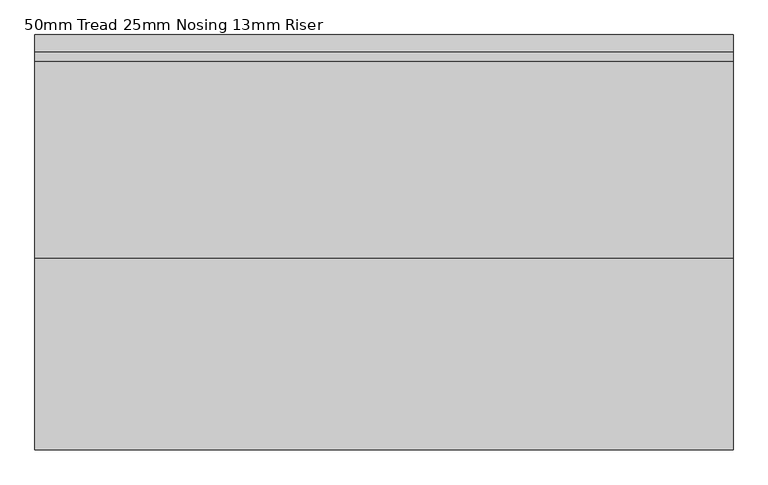
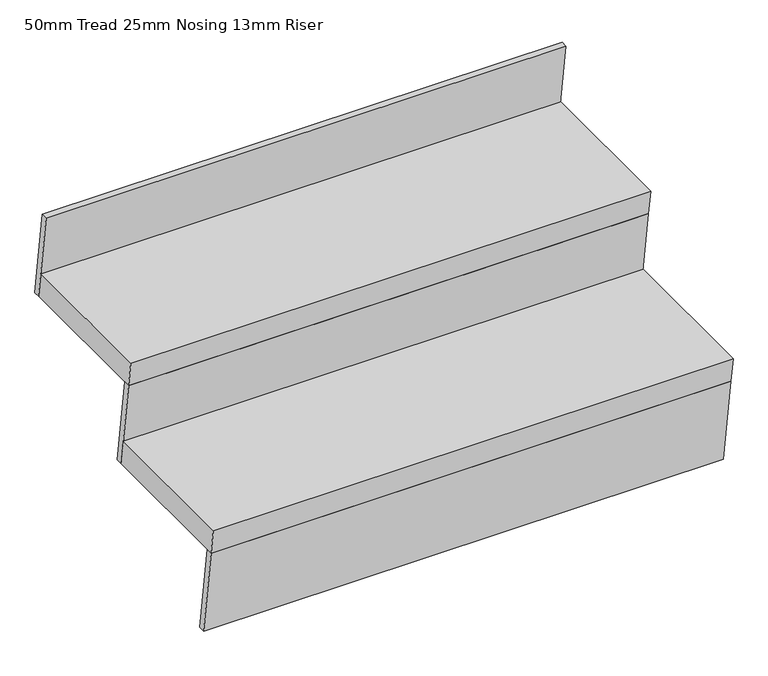
"""IFC4 building model written with IfcOpenShell, lengths in millimetres: stair flight geometry, 50mm Tread 25mm Nosing 13mm Riser."""

from ifc_helpers import new_model, si_unit, frame, origin, place, context, project, spatial, polyline, outline, extrude, source, transform, mapped, element, save


def stair_flight_50mm_tread_25mm_nosing_13mm_riser_775a8025(model_context):
    return source(origin(), model_context, "Body", "SweptSolid", [
        extrude(outline(polyline([(7333.8660835, 1217.3913043), (7633.8660835, 1217.3913043), (7641.0535835, 1167.3913043), (7341.0535835, 1167.3913043), (7333.8660835, 1217.3913043)])), frame((-12602.0787807, 0.0, 0.0), z_axis=(1.0, 0.0, 0.0), x_axis=(0.0, 1.0, 0.0)), (0.0, 0.0, 1.0), 1000.0257812),
        extrude(outline(polyline([(7341.0535835, 1167.3913043), (7353.6820735, 1167.3913043), (7378.6820735, 993.4782609), (7366.0535835, 993.4782609), (7341.0535835, 1167.3913043)])), frame((-12602.0787807, 0.0, 0.0), z_axis=(1.0, 0.0, 0.0), x_axis=(0.0, 1.0, 0.0)), (0.0, 0.0, 1.0), 1000.0257813),
        extrude(outline(polyline([(7616.0535835, 1341.3043478), (7628.6820735, 1341.3043478), (7653.6820735, 1167.3913043), (7641.0535835, 1167.3913043), (7616.0535835, 1341.3043478)])), frame((-12602.0787807, 0.0, 0.0), z_axis=(1.0, 0.0, 0.0), x_axis=(0.0, 1.0, 0.0)), (0.0, 0.0, 1.0), 1000.0257813),
        extrude(outline(polyline([(7891.0535835, 1515.2173913), (7903.6820735, 1515.2173913), (7928.6820735, 1341.3043478), (7916.0535835, 1341.3043478), (7891.0535835, 1515.2173913)])), frame((-12602.0787807, 0.0, 0.0), z_axis=(1.0, 0.0, 0.0), x_axis=(0.0, 1.0, 0.0)), (0.0, 0.0, 1.0), 1000.0257813),
        extrude(outline(polyline([(7608.8660835, 1391.3043478), (7908.8660835, 1391.3043478), (7916.0535835, 1341.3043478), (7616.0535835, 1341.3043478), (7608.8660835, 1391.3043478)])), frame((-12602.0787807, 0.0, 0.0), z_axis=(1.0, 0.0, 0.0), x_axis=(0.0, 1.0, 0.0)), (0.0, 0.0, 1.0), 1000.0257812),
    ])


if __name__ == "__main__":
    model = new_model("IFC4")
    model_context = context("Model", 3, world=origin())
    ifc_project = project(units=[si_unit("LENGTHUNIT", "METRE", prefix="MILLI")], contexts=[model_context])
    site = spatial("IfcSite", under=ifc_project)
    building = spatial("IfcBuilding", under=site)
    placement = place(None, origin())
    stair_flight_50mm_tread_25mm_nosing_13mm_riser_shape = stair_flight_50mm_tread_25mm_nosing_13mm_riser_775a8025(model_context)
    element("IfcStairFlight", 1, ObjectType="50mm Tread 25mm Nosing 13mm Riser", at=placement, inside=building, context=model_context, shape_type="MappedRepresentation", body=[
        mapped(stair_flight_50mm_tread_25mm_nosing_13mm_riser_shape, transform((0.0, 0.0, 0.0), x_axis=(1.0, 0.0, 0.0), y_axis=(0.0, 1.0, 0.0), z_axis=(0.0, 0.0, 1.0))),
    ])
    save(model, "model.ifc")
